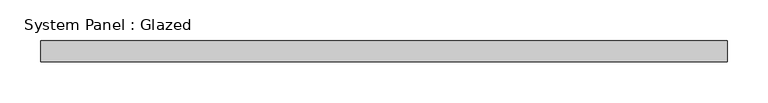
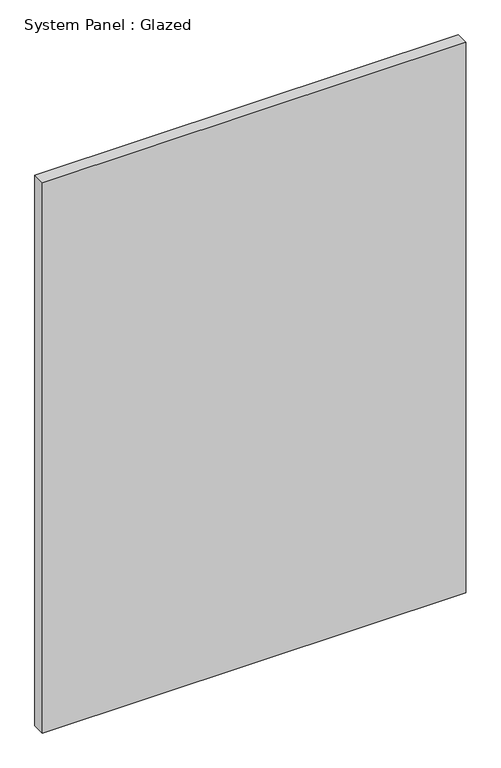
"""IFC4 building model written with IfcOpenShell, lengths in millimetres: plate geometry, System Panel : Glazed."""

from ifc_helpers import new_model, si_unit, origin, origin_with_axes, place, context, project, spatial, polyline, outline, extrude, source, transform, mapped, element, save


def system_panel_glazed_59c8d2f2(model_context):
    return source(origin(), model_context, "Body", "SweptSolid", [
        extrude(outline(polyline([(420.5054332, 19.05), (-420.5054332, 19.05), (-420.5054332, 44.45), (420.5054332, 44.45), (420.5054332, 19.05)])), origin_with_axes(), (0.0, 0.0, 1.0), 1155.7),
    ])


if __name__ == "__main__":
    model = new_model("IFC4")
    model_context = context("Model", 3, world=origin())
    ifc_project = project(units=[si_unit("LENGTHUNIT", "METRE", prefix="MILLI")], contexts=[model_context])
    site = spatial("IfcSite", under=ifc_project)
    building = spatial("IfcBuilding", under=site)
    placement = place(None, origin())
    system_panel_glazed_shape = system_panel_glazed_59c8d2f2(model_context)
    element("IfcPlate", 1, ObjectType="System Panel : Glazed", at=placement, inside=building, context=model_context, shape_type="MappedRepresentation", body=[
        mapped(system_panel_glazed_shape, transform((0.0, 0.0, 0.0), x_axis=(1.0, 0.0, 0.0), y_axis=(0.0, 1.0, 0.0), z_axis=(0.0, 0.0, 1.0))),
    ])
    save(model, "model.ifc")

# Revit data of these elements
# Type "System Panel : Glazed"
#   Construction Type Id = "GSP4R"
#   Analytic Construction = "1/8 in Pilkington single glazing"
#   Visual Light Transmittance = 0.9
#   Solar Heat Gain Coefficient = 0.86
#   Heat Transfer Coefficient (U) = 1.18115 BTU/(h·ft²·°F)
# Element 1 (IfcPlate, "System Panel : Glazed")
#   Materials on its faces: "Glass"
# Materials
#   "Glass": class "Glass", colour RGB 0 128 192, transparency 0.75, Description = "Soda Lime Glass", Cost = 0
